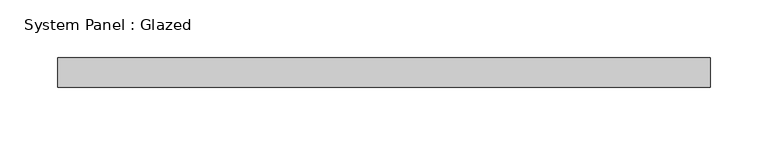
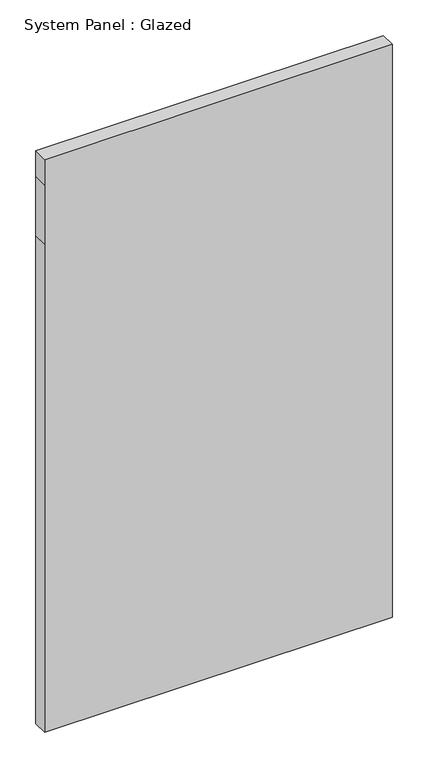
"""IFC4 building model written with IfcOpenShell, lengths in millimetres: plate geometry, System Panel : Glazed."""

from ifc_helpers import new_model, si_unit, frame, origin, place, context, project, spatial, polyline, outline, extrude, source, transform, mapped, element, save


def system_panel_glazed_3a936e0b(model_context):
    return source(origin(), model_context, "Body", "SweptSolid", [
        extrude(outline(polyline([(0.0, -282.575), (0.0, 282.575), (839.0301773, 282.575), (940.6301773, 282.575), (985.0801773, 282.575), (985.0801773, -282.575), (940.6301773, -282.575), (839.0301773, -282.575), (0.0, -282.575)])), frame((0.0, 19.05, 0.0), z_axis=(0.0, 1.0, 0.0), x_axis=(0.0, 0.0, 1.0)), (0.0, 0.0, 1.0), 25.4),
    ])


if __name__ == "__main__":
    model = new_model("IFC4")
    model_context = context("Model", 3, world=origin())
    ifc_project = project(units=[si_unit("LENGTHUNIT", "METRE", prefix="MILLI")], contexts=[model_context])
    site = spatial("IfcSite", under=ifc_project)
    building = spatial("IfcBuilding", under=site)
    placement = place(None, origin())
    system_panel_glazed_shape = system_panel_glazed_3a936e0b(model_context)
    element("IfcPlate", 1, ObjectType="System Panel : Glazed", at=placement, inside=building, context=model_context, shape_type="MappedRepresentation", body=[
        mapped(system_panel_glazed_shape, transform((0.0, 0.0, 0.0), x_axis=(1.0, 0.0, 0.0), y_axis=(0.0, 1.0, 0.0), z_axis=(0.0, 0.0, 1.0))),
    ])
    save(model, "model.ifc")

# Revit data of these elements
# Type "System Panel : Glazed"
#   Construction Type Id = "GSP4R"
#   Analytic Construction = "1/8 in Pilkington single glazing"
#   Visual Light Transmittance = 0.9
#   Solar Heat Gain Coefficient = 0.86
#   Heat Transfer Coefficient (U) = 1.18115 BTU/(h·ft²·°F)
#   Define Thermal Properties by = 1
# Element 1 (IfcPlate, "System Panel : Glazed")
#   Materials on its faces: "Glass"
# Materials
#   "Glass": class "Glass", colour RGB 0 128 192, transparency 0.75, Description = "Soda Lime Glass", Cost = 0
